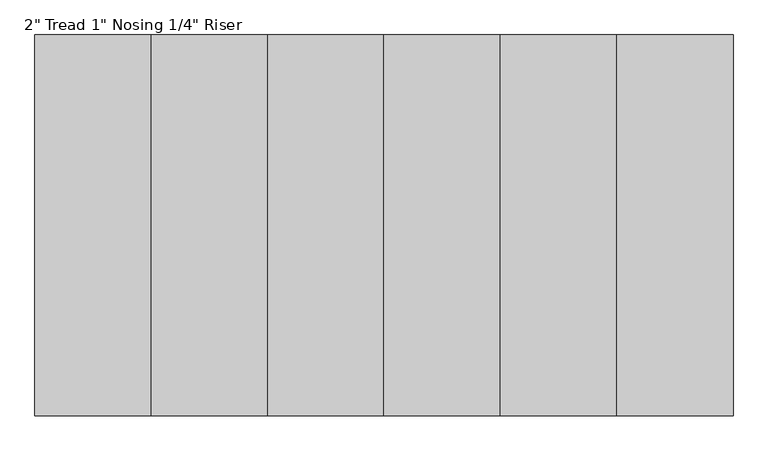
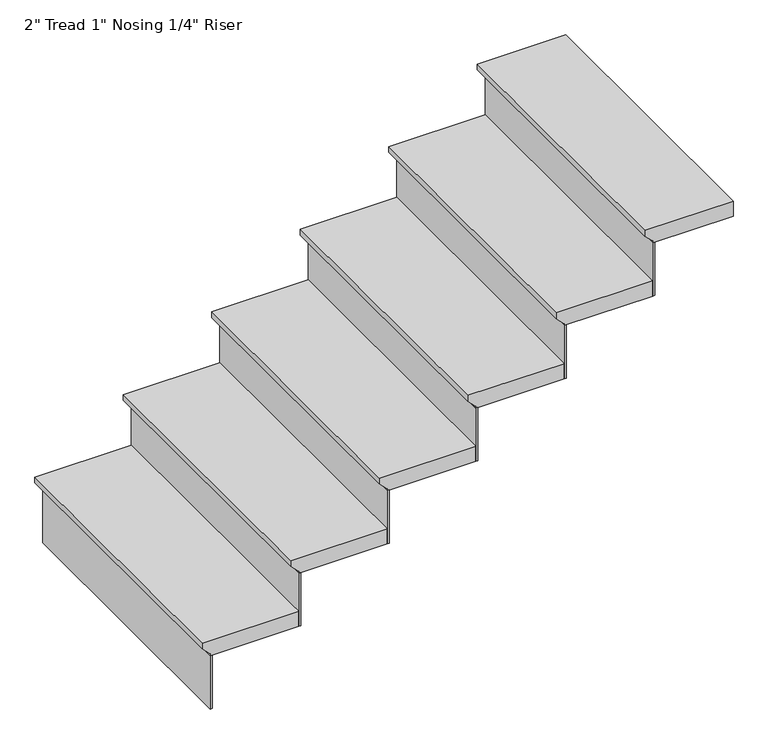
"""IFC4 building model written with IfcOpenShell, lengths in millimetres: stair flight geometry."""

from ifc_helpers import new_model, si_unit, frame, origin, place, context, project, spatial, polyline, outline, extrude, source, transform, mapped, element, save


def stair_flight_7eff537e(model_context):
    return source(origin(), model_context, "Body", "SweptSolid", [
        extrude(outline(polyline([(2133.6, 10858.7752377), (2133.6, 10553.9752377), (2114.55, 10553.9752377), (2089.15, 10579.3752377), (2082.8, 10579.3752377), (2082.8, 10858.7752377), (2133.6, 10858.7752377)])), frame((0.0, 22006.2919009, 0.0), z_axis=(0.0, 1.0, 0.0), x_axis=(0.0, 0.0, 1.0)), (0.0, 0.0, 1.0), 914.4),
        extrude(outline(polyline([(10585.7252377, 22006.2919009), (10579.3752377, 22006.2919009), (10579.3752377, 22920.6919009), (10585.7252377, 22920.6919009), (10585.7252377, 22006.2919009)])), frame((0.0, 0.0, 1905.0), z_axis=(0.0, 0.0, 1.0), x_axis=(1.0, 0.0, 0.0)), (0.0, 0.0, 1.0), 177.8),
        extrude(outline(polyline([(10865.1252377, 22006.2919009), (10858.7752377, 22006.2919009), (10858.7752377, 22920.6919009), (10865.1252377, 22920.6919009), (10865.1252377, 22006.2919009)])), frame((0.0, 0.0, 2082.8), z_axis=(0.0, 0.0, 1.0), x_axis=(1.0, 0.0, 0.0)), (0.0, 0.0, 1.0), 177.8),
        extrude(outline(polyline([(2311.4, 11138.1752377), (2311.4, 10833.3752377), (2292.35, 10833.3752377), (2266.95, 10858.7752377), (2260.6, 10858.7752377), (2260.6, 11138.1752377), (2311.4, 11138.1752377)])), frame((0.0, 22006.2919009, 0.0), z_axis=(0.0, 1.0, 0.0), x_axis=(0.0, 0.0, 1.0)), (0.0, 0.0, 1.0), 914.4),
        extrude(outline(polyline([(11144.5252377, 22006.2919009), (11138.1752377, 22006.2919009), (11138.1752377, 22920.6919009), (11144.5252377, 22920.6919009), (11144.5252377, 22006.2919009)])), frame((0.0, 0.0, 2260.6), z_axis=(0.0, 0.0, 1.0), x_axis=(1.0, 0.0, 0.0)), (0.0, 0.0, 1.0), 177.8),
        extrude(outline(polyline([(2489.2, 11417.5752377), (2489.2, 11112.7752377), (2470.15, 11112.7752377), (2444.75, 11138.1752377), (2438.4, 11138.1752377), (2438.4, 11417.5752377), (2489.2, 11417.5752377)])), frame((0.0, 22006.2919009, 0.0), z_axis=(0.0, 1.0, 0.0), x_axis=(0.0, 0.0, 1.0)), (0.0, 0.0, 1.0), 914.4),
        extrude(outline(polyline([(11423.9252377, 22006.2919009), (11417.5752377, 22006.2919009), (11417.5752377, 22920.6919009), (11423.9252377, 22920.6919009), (11423.9252377, 22006.2919009)])), frame((0.0, 0.0, 2438.4), z_axis=(0.0, 0.0, 1.0), x_axis=(1.0, 0.0, 0.0)), (0.0, 0.0, 1.0), 177.8),
        extrude(outline(polyline([(2667.0, 11696.9752377), (2667.0, 11392.1752377), (2647.95, 11392.1752377), (2622.55, 11417.5752377), (2616.2, 11417.5752377), (2616.2, 11696.9752377), (2667.0, 11696.9752377)])), frame((0.0, 22006.2919009, 0.0), z_axis=(0.0, 1.0, 0.0), x_axis=(0.0, 0.0, 1.0)), (0.0, 0.0, 1.0), 914.4),
        extrude(outline(polyline([(11703.3252377, 22006.2919009), (11696.9752377, 22006.2919009), (11696.9752377, 22920.6919009), (11703.3252377, 22920.6919009), (11703.3252377, 22006.2919009)])), frame((0.0, 0.0, 2616.2), z_axis=(0.0, 0.0, 1.0), x_axis=(1.0, 0.0, 0.0)), (0.0, 0.0, 1.0), 177.8),
        extrude(outline(polyline([(2844.8, 11976.3752377), (2844.8, 11671.5752377), (2825.75, 11671.5752377), (2800.35, 11696.9752377), (2794.0, 11696.9752377), (2794.0, 11976.3752377), (2844.8, 11976.3752377)])), frame((0.0, 22006.2919009, 0.0), z_axis=(0.0, 1.0, 0.0), x_axis=(0.0, 0.0, 1.0)), (0.0, 0.0, 1.0), 914.4),
        extrude(outline(polyline([(11982.7252377, 22006.2919009), (11976.3752377, 22006.2919009), (11976.3752377, 22920.6919009), (11982.7252377, 22920.6919009), (11982.7252377, 22006.2919009)])), frame((0.0, 0.0, 2794.0), z_axis=(0.0, 0.0, 1.0), x_axis=(1.0, 0.0, 0.0)), (0.0, 0.0, 1.0), 177.8),
        extrude(outline(polyline([(3022.6, 12230.3752377), (3022.6, 11950.9752377), (3003.55, 11950.9752377), (2978.15, 11976.3752377), (2971.8, 11976.3752377), (2971.8, 12230.3752377), (3022.6, 12230.3752377)])), frame((0.0, 22006.2919009, 0.0), z_axis=(0.0, 1.0, 0.0), x_axis=(0.0, 0.0, 1.0)), (0.0, 0.0, 1.0), 914.4),
    ])


if __name__ == "__main__":
    model = new_model("IFC4")
    model_context = context("Model", 3, world=origin())
    ifc_project = project(units=[si_unit("LENGTHUNIT", "METRE", prefix="MILLI")], contexts=[model_context])
    site = spatial("IfcSite", under=ifc_project)
    building = spatial("IfcBuilding", under=site)
    placement = place(None, origin())
    stair_flight_shape = stair_flight_7eff537e(model_context)
    element("IfcStairFlight", 1, ObjectType="2\" Tread 1\" Nosing 1/4\" Riser", at=placement, inside=building, context=model_context, shape_type="MappedRepresentation", body=[
        mapped(stair_flight_shape, transform((0.0, 0.0, 0.0), x_axis=(1.0, 0.0, 0.0), y_axis=(0.0, 1.0, 0.0), z_axis=(0.0, 0.0, 1.0))),
    ])
    save(model, "model.ifc")
